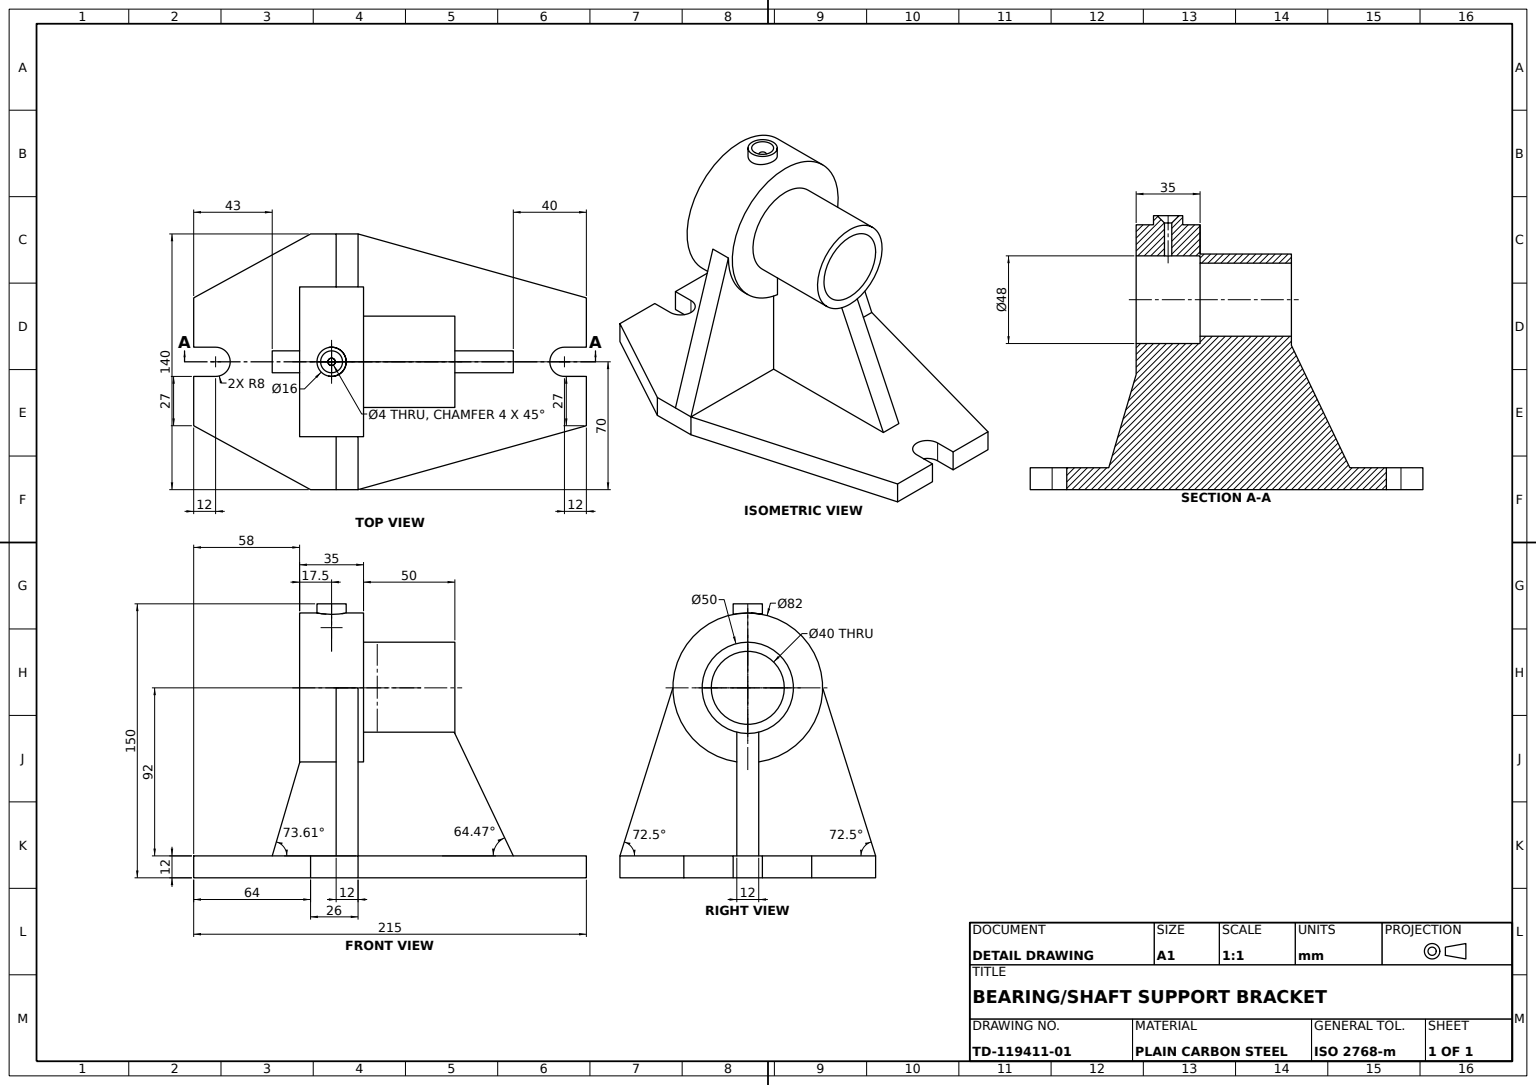
from build123d import *

# Parameters (mm, degrees)
BASE_PLATE_DEPTH              = 12
SUPPORT_WEB_DEPTH             = 12
WEB_GUSSET_RIB_REACH          = 205.838
WEB_GUSSET_RIB_SKETCH_WALL_W  = 462.836477652
WEB_GUSSET_RIB_SKETCH_WALL_H  = 12
SIDE_GUSSET_RIB_REACH         = 205.838
SIDE_GUSSET_RIB_SKETCH_WALL_W = 483.925921336
SIDE_GUSSET_RIB_SKETCH_WALL_H = 12
GREASE_BOSS_16_REACH          = 209.425
GREASE_BOSS_16_END_RADIUS     = 41
GREASE_BOSS_SKETCH_R          = 8
LUBE_HOLE_SKETCH_R            = 2
LUBE_HOLE_DEPTH               = 35
GREASE_BOSS_CHAMFER_4X45_SIZE = 4


with BuildPart() as part:
    # Base Plate Sketch → Base Plate (new body)
    with BuildSketch(Plane(origin=(0, 0, 0), x_dir=(1, 0, 0), z_dir=(0, 1, 0))):
        with BuildLine():
            Line((-90, -35), (-90, -8))
            Line((-90, -8), (-78, -8))
            ThreePointArc((-78, -8), (-70, 0), (-78, 8))
            Line((-78, 8), (-90, 8))
            Line((-90, 8), (-90, 35))
            Line((-90, 35), (-26, 70))
            Line((-26, 70), (0, 70))
            Line((0, 70), (125, 35))
            Line((125, 35), (125, 8))
            Line((125, 8), (113, 8))
            ThreePointArc((113, 8), (105, 0), (113, -8))
            Line((113, -8), (125, -8))
            Line((125, -8), (125, -35))
            Line((125, -35), (0, -70))
            Line((0, -70), (-26, -70))
            Line((-26, -70), (-90, -35))
        make_face()
    extrude(amount=BASE_PLATE_DEPTH)



with BuildPart() as body_2:
    # Bearing Boss Profile → Bearing Boss (revolve)
    with BuildSketch(Plane.XY, mode=Mode.PRIVATE) as bearing_boss_sk:
        Polygon((53, 104), (-32, 104), (-32, 63), (3, 63), (3, 79), (53, 79), align=None)
    revolve(bearing_boss_sk.sketch.rotate(Axis((53, 104, 0), (-1, 0, 0)), 180), axis=Axis((53, 104, 0), (-1, 0, 0)))

    # Stepped Bore Profile → Stepped Bore (revolve, cut)
    with BuildSketch(Plane.XY, mode=Mode.PRIVATE) as stepped_bore_sk:
        Polygon((-32, 128), (3, 128), (3, 124), (53, 124), (53, 104), (-32, 104), align=None)
    revolve(stepped_bore_sk.sketch.rotate(Axis((-32, 104, 0), (1, 0, 0)), 90), axis=Axis((-32, 104, 0), (1, 0, 0)), mode=Mode.SUBTRACT)


with BuildPart() as part_1:
    add(part.part)

    add(body_2.part)  # Support Web merges body 2
    # Support Web Sketch → Support Web (add)
    with BuildSketch(Plane(origin=(0, 0, 0), x_dir=(0, 0, -1), z_dir=(1, 0, 0))):
        with BuildLine():
            Line((-70, 12), (-41, 104))
            ThreePointArc((-41, 104), (0, 63), (41, 104))
            Line((41, 104), (70, 12))
            Line((70, 12), (35, 12))
            Line((35, 12), (8, 12))
            Line((8, 12), (-8, 12))
            Line((-8, 12), (-35, 12))
            Line((-35, 12), (-70, 12))
        make_face()
    extrude(amount=-SUPPORT_WEB_DEPTH)

    # Web Gusset Rib Sketch wall → Web Gusset Rib (add, up to next)
    with BuildSketch(Plane(origin=(-39.5, 37.5, 0), x_dir=(-0.282166323992, -0.959365501571, 0), z_dir=(0.959365501571, -0.282166323992, 0)), mode=Mode.PRIVATE) as web_gusset_rib_sk1:
        Rectangle(WEB_GUSSET_RIB_SKETCH_WALL_W, WEB_GUSSET_RIB_SKETCH_WALL_H)
    web_gusset_rib_tool1 = extrude(web_gusset_rib_sk1.sketch, amount=WEB_GUSSET_RIB_REACH, mode=Mode.PRIVATE) - part_1.part
    add(web_gusset_rib_tool1.solids().sort_by_distance((-39.5, 37.5, 0))[0])

    # Side Gusset Rib Sketch wall → Side Gusset Rib (add, up to next)
    with BuildSketch(Plane(origin=(69, 45.5, 0), x_dir=(0.430978873925, -0.90236201728, 0), z_dir=(0.90236201728, 0.430978873925, 0)), mode=Mode.PRIVATE) as side_gusset_rib_sk1:
        Rectangle(SIDE_GUSSET_RIB_SKETCH_WALL_W, SIDE_GUSSET_RIB_SKETCH_WALL_H)
    side_gusset_rib_tool1 = extrude(side_gusset_rib_sk1.sketch, amount=-SIDE_GUSSET_RIB_REACH, mode=Mode.PRIVATE) - part_1.part
    add(side_gusset_rib_tool1.solids().sort_by_distance((69, 45.5, 0))[0])

    # Grease Boss Ø16: up to this cylinder (the profile starts outside it)
    grease_boss_16_end = Plane(origin=(-14.5, 104, 0), z_dir=(1, 0, 0)) * Cylinder(GREASE_BOSS_16_END_RADIUS, 501.85, mode=Mode.PRIVATE)
    # Grease Boss Sketch → Grease Boss Ø16 (add, up to the surface)
    with BuildSketch(Plane(origin=(0, 150, 0), x_dir=(1, 0, 0), z_dir=(0, 1, 0)), mode=Mode.PRIVATE) as grease_boss_16_sk1:
        with Locations(Location((-14.5, 0, 0), (0, 0, 270))):
            Circle(GREASE_BOSS_SKETCH_R)
    grease_boss_16_tool1 = extrude(grease_boss_16_sk1.sketch, amount=-GREASE_BOSS_16_REACH, mode=Mode.PRIVATE) - grease_boss_16_end
    add(grease_boss_16_tool1.solids().sort_by_distance((-14.5, 150, 0))[0])

    # Lube Hole Sketch → Lube Hole (cut)
    with BuildSketch(Plane(origin=(0, 150, 0), x_dir=(1, 0, 0), z_dir=(0, 1, 0))):
        with Locations(Location((-14.5, 0, 0), (0, 0, 270))):
            Circle(LUBE_HOLE_SKETCH_R)
    extrude(amount=-LUBE_HOLE_DEPTH, mode=Mode.SUBTRACT)

    # Grease Boss Chamfer 4x45°
    grease_boss_chamfer_4x45_edges = [part_1.edges().sort_by_distance(p)[0] for p in [
        (-14.5, 150, -2),
    ]]
    chamfer(grease_boss_chamfer_4x45_edges, length=GREASE_BOSS_CHAMFER_4X45_SIZE)


solid = part_1.part
